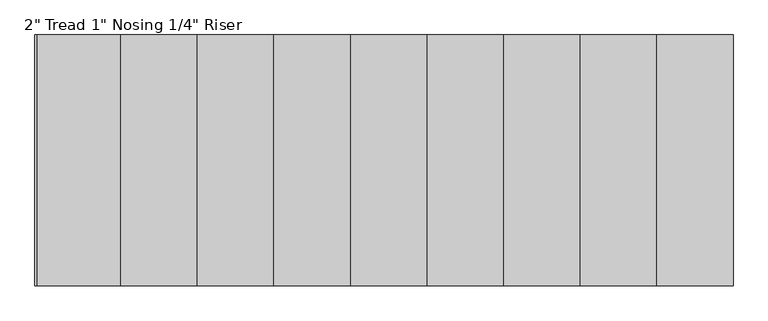
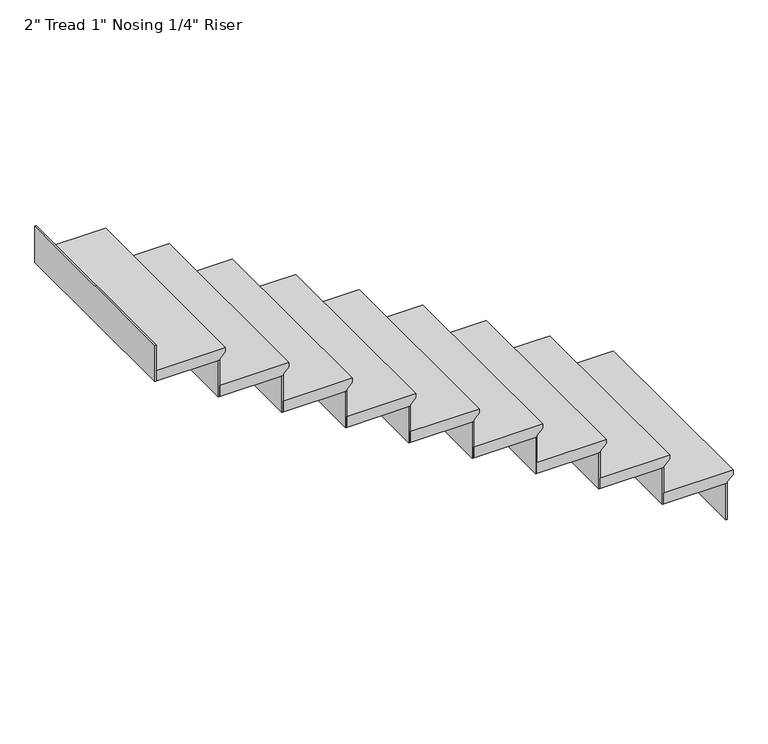
"""IFC4 building model written with IfcOpenShell, lengths in millimetres: stair flight geometry."""

from ifc_helpers import new_model, si_unit, frame, origin, place, context, project, spatial, polyline, outline, extrude, source, transform, mapped, element, save


def stair_flight_b4d473f5(model_context):
    return source(origin(), model_context, "Body", "SweptSolid", [
        extrude(outline(polyline([(1693.3333333, -6294.6389568), (1693.3333333, -6599.4389568), (1642.5333333, -6599.4389568), (1642.5333333, -6320.0389568), (1648.8833333, -6320.0389568), (1674.2833333, -6294.6389568), (1693.3333333, -6294.6389568)])), frame((0.0, 2281.1342758, 0.0), z_axis=(0.0, 1.0, 0.0), x_axis=(0.0, 0.0, 1.0)), (0.0, 0.0, 1.0), 914.4),
        extrude(outline(polyline([(-6326.3889568, 3195.5342758), (-6320.0389568, 3195.5342758), (-6320.0389568, 2281.1342758), (-6326.3889568, 2281.1342758), (-6326.3889568, 3195.5342758)])), frame((0.0, 0.0, 1473.2), z_axis=(0.0, 0.0, 1.0), x_axis=(1.0, 0.0, 0.0)), (0.0, 0.0, 1.0), 169.3333333),
        extrude(outline(polyline([(-6605.7889568, 3195.5342758), (-6599.4389568, 3195.5342758), (-6599.4389568, 2281.1342758), (-6605.7889568, 2281.1342758), (-6605.7889568, 3195.5342758)])), frame((0.0, 0.0, 1642.5333333), z_axis=(0.0, 0.0, 1.0), x_axis=(1.0, 0.0, 0.0)), (0.0, 0.0, 1.0), 169.3333333),
        extrude(outline(polyline([(1862.6666667, -6574.0389568), (1862.6666667, -6878.8389568), (1811.8666667, -6878.8389568), (1811.8666667, -6599.4389568), (1818.2166667, -6599.4389568), (1843.6166667, -6574.0389568), (1862.6666667, -6574.0389568)])), frame((0.0, 2281.1342758, 0.0), z_axis=(0.0, 1.0, 0.0), x_axis=(0.0, 0.0, 1.0)), (0.0, 0.0, 1.0), 914.4),
        extrude(outline(polyline([(-6885.1889568, 3195.5342758), (-6878.8389568, 3195.5342758), (-6878.8389568, 2281.1342758), (-6885.1889568, 2281.1342758), (-6885.1889568, 3195.5342758)])), frame((0.0, 0.0, 1811.8666667), z_axis=(0.0, 0.0, 1.0), x_axis=(1.0, 0.0, 0.0)), (0.0, 0.0, 1.0), 169.3333333),
        extrude(outline(polyline([(2032.0, -6853.4389568), (2032.0, -7158.2389568), (1981.2, -7158.2389568), (1981.2, -6878.8389568), (1987.55, -6878.8389568), (2012.95, -6853.4389568), (2032.0, -6853.4389568)])), frame((0.0, 2281.1342758, 0.0), z_axis=(0.0, 1.0, 0.0), x_axis=(0.0, 0.0, 1.0)), (0.0, 0.0, 1.0), 914.4),
        extrude(outline(polyline([(-7164.5889568, 3195.5342758), (-7158.2389568, 3195.5342758), (-7158.2389568, 2281.1342758), (-7164.5889568, 2281.1342758), (-7164.5889568, 3195.5342758)])), frame((0.0, 0.0, 1981.2), z_axis=(0.0, 0.0, 1.0), x_axis=(1.0, 0.0, 0.0)), (0.0, 0.0, 1.0), 169.3333333),
        extrude(outline(polyline([(2201.3333333, -7132.8389568), (2201.3333333, -7437.6389568), (2150.5333333, -7437.6389568), (2150.5333333, -7158.2389568), (2156.8833333, -7158.2389568), (2182.2833333, -7132.8389568), (2201.3333333, -7132.8389568)])), frame((0.0, 2281.1342758, 0.0), z_axis=(0.0, 1.0, 0.0), x_axis=(0.0, 0.0, 1.0)), (0.0, 0.0, 1.0), 914.4),
        extrude(outline(polyline([(-7443.9889568, 3195.5342758), (-7437.6389568, 3195.5342758), (-7437.6389568, 2281.1342758), (-7443.9889568, 2281.1342758), (-7443.9889568, 3195.5342758)])), frame((0.0, 0.0, 2150.5333333), z_axis=(0.0, 0.0, 1.0), x_axis=(1.0, 0.0, 0.0)), (0.0, 0.0, 1.0), 169.3333333),
        extrude(outline(polyline([(2370.6666667, -7412.2389568), (2370.6666667, -7717.0389568), (2319.8666667, -7717.0389568), (2319.8666667, -7437.6389568), (2326.2166667, -7437.6389568), (2351.6166667, -7412.2389568), (2370.6666667, -7412.2389568)])), frame((0.0, 2281.1342758, 0.0), z_axis=(0.0, 1.0, 0.0), x_axis=(0.0, 0.0, 1.0)), (0.0, 0.0, 1.0), 914.4),
        extrude(outline(polyline([(-7723.3889568, 3195.5342758), (-7717.0389568, 3195.5342758), (-7717.0389568, 2281.1342758), (-7723.3889568, 2281.1342758), (-7723.3889568, 3195.5342758)])), frame((0.0, 0.0, 2319.8666667), z_axis=(0.0, 0.0, 1.0), x_axis=(1.0, 0.0, 0.0)), (0.0, 0.0, 1.0), 169.3333333),
        extrude(outline(polyline([(2540.0, -7691.6389568), (2540.0, -7996.4389568), (2489.2, -7996.4389568), (2489.2, -7717.0389568), (2495.55, -7717.0389568), (2520.95, -7691.6389568), (2540.0, -7691.6389568)])), frame((0.0, 2281.1342758, 0.0), z_axis=(0.0, 1.0, 0.0), x_axis=(0.0, 0.0, 1.0)), (0.0, 0.0, 1.0), 914.4),
        extrude(outline(polyline([(-8002.7889568, 3195.5342758), (-7996.4389568, 3195.5342758), (-7996.4389568, 2281.1342758), (-8002.7889568, 2281.1342758), (-8002.7889568, 3195.5342758)])), frame((0.0, 0.0, 2489.2), z_axis=(0.0, 0.0, 1.0), x_axis=(1.0, 0.0, 0.0)), (0.0, 0.0, 1.0), 169.3333333),
        extrude(outline(polyline([(2709.3333333, -7971.0389568), (2709.3333333, -8275.8389568), (2658.5333333, -8275.8389568), (2658.5333333, -7996.4389568), (2664.8833333, -7996.4389568), (2690.2833333, -7971.0389568), (2709.3333333, -7971.0389568)])), frame((0.0, 2281.1342758, 0.0), z_axis=(0.0, 1.0, 0.0), x_axis=(0.0, 0.0, 1.0)), (0.0, 0.0, 1.0), 914.4),
        extrude(outline(polyline([(-8282.1889568, 3195.5342758), (-8275.8389568, 3195.5342758), (-8275.8389568, 2281.1342758), (-8282.1889568, 2281.1342758), (-8282.1889568, 3195.5342758)])), frame((0.0, 0.0, 2658.5333333), z_axis=(0.0, 0.0, 1.0), x_axis=(1.0, 0.0, 0.0)), (0.0, 0.0, 1.0), 169.3333333),
        extrude(outline(polyline([(2878.6666667, -8250.4389568), (2878.6666667, -8555.2389568), (2827.8666667, -8555.2389568), (2827.8666667, -8275.8389568), (2834.2166667, -8275.8389568), (2859.6166667, -8250.4389568), (2878.6666667, -8250.4389568)])), frame((0.0, 2281.1342758, 0.0), z_axis=(0.0, 1.0, 0.0), x_axis=(0.0, 0.0, 1.0)), (0.0, 0.0, 1.0), 914.4),
        extrude(outline(polyline([(-8561.5889568, 3195.5342758), (-8555.2389568, 3195.5342758), (-8555.2389568, 2281.1342758), (-8561.5889568, 2281.1342758), (-8561.5889568, 3195.5342758)])), frame((0.0, 0.0, 2827.8666667), z_axis=(0.0, 0.0, 1.0), x_axis=(1.0, 0.0, 0.0)), (0.0, 0.0, 1.0), 169.3333333),
        extrude(outline(polyline([(-8840.9889568, 3195.5342758), (-8834.6389568, 3195.5342758), (-8834.6389568, 2281.1342758), (-8840.9889568, 2281.1342758), (-8840.9889568, 3195.5342758)])), frame((0.0, 0.0, 2997.2), z_axis=(0.0, 0.0, 1.0), x_axis=(1.0, 0.0, 0.0)), (0.0, 0.0, 1.0), 169.3333333),
        extrude(outline(polyline([(3048.0, -8529.8389568), (3048.0, -8834.6389568), (2997.2, -8834.6389568), (2997.2, -8555.2389568), (3003.55, -8555.2389568), (3028.95, -8529.8389568), (3048.0, -8529.8389568)])), frame((0.0, 2281.1342758, 0.0), z_axis=(0.0, 1.0, 0.0), x_axis=(0.0, 0.0, 1.0)), (0.0, 0.0, 1.0), 914.4),
    ])


if __name__ == "__main__":
    model = new_model("IFC4")
    model_context = context("Model", 3, world=origin())
    ifc_project = project(units=[si_unit("LENGTHUNIT", "METRE", prefix="MILLI")], contexts=[model_context])
    site = spatial("IfcSite", under=ifc_project)
    building = spatial("IfcBuilding", under=site)
    placement = place(None, origin())
    stair_flight_shape = stair_flight_b4d473f5(model_context)
    element("IfcStairFlight", 1, ObjectType="2\" Tread 1\" Nosing 1/4\" Riser", at=placement, inside=building, context=model_context, shape_type="MappedRepresentation", body=[
        mapped(stair_flight_shape, transform((0.0, 0.0, 0.0), x_axis=(1.0, 0.0, 0.0), y_axis=(0.0, 1.0, 0.0), z_axis=(0.0, 0.0, 1.0))),
    ])
    save(model, "model.ifc")
